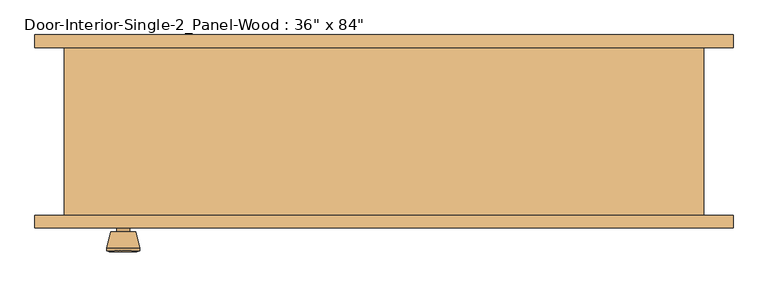
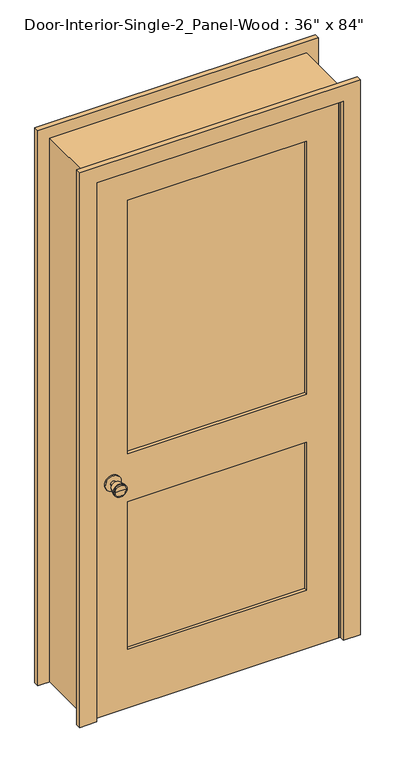
"""IFC4 building model written with IfcOpenShell, lengths in millimetres: door geometry."""

from ifc_helpers import new_model, si_unit, point, frame, frame_2d, origin, place, context, project, spatial, polyline, circle_curve, trimmed, segment, composite_curve, outline, extrude, faceted_brep, source, transform, mapped, element, save
from ifc_brep_helpers import plane_surface, cylinder_surface, revolved_surface, advanced_brep


def door_acb80719(model_context):
    return source(origin(), model_context, "Body", "SolidModel", [
        advanced_brep(
        [(-393.7, -82.9, 914.4), (-403.7, -82.9, 914.4), (-383.7, -82.9, 914.4), (-373.2241324, -33.9, 914.4), (-414.1758676, -33.9, 914.4), (-393.7, -33.9, 914.4), (-368.7, -35.7278681, 914.4), (-418.7, -35.7278681, 914.4), (-368.7, -39.1915463, 914.4), (-418.7, -39.1915463, 914.4), (-375.063764, -63.9, 914.4), (-412.336236, -63.9, 914.4), (-383.7, -63.9, 914.4), (-403.7, -63.9, 914.4)],
        [
            (0, 1),
            (1, 2, circle_curve(frame((-393.7, -82.9, 914.4), z_axis=(0.0, -1.0, 0.0), x_axis=(-1.0, 0.0, 0.0)), 10.0)),
            (2, 0),
            (2, 1, circle_curve(frame((-393.7, -82.9, 914.4), z_axis=(0.0, -1.0, 0.0), x_axis=(-1.0, 0.0, 0.0)), 10.0)),
            (3, 4, circle_curve(frame((-393.7, -33.9, 914.4), z_axis=(0.0, 1.0, 0.0), x_axis=(-1.0, 0.0, 0.0)), 20.4758676)),
            (4, 5),
            (5, 3),
            (4, 3, circle_curve(frame((-393.7, -33.9, 914.4), z_axis=(0.0, 1.0, 0.0), x_axis=(-1.0, 0.0, 0.0)), 20.4758676)),
            (6, 7, circle_curve(frame((-393.7, -35.7278681, 914.4), z_axis=(0.0, 1.0, 0.0), x_axis=(-1.0, 0.0, 0.0)), 25.0)),
            (7, 4),
            (3, 6),
            (7, 6, circle_curve(frame((-393.7, -35.7278681, 914.4), z_axis=(0.0, 1.0, 0.0), x_axis=(-1.0, 0.0, 0.0)), 25.0)),
            (8, 9, circle_curve(frame((-393.7, -39.1915463, 914.4), z_axis=(0.0, 1.0, 0.0), x_axis=(-1.0, 0.0, 0.0)), 25.0)),
            (9, 7),
            (6, 8),
            (9, 8, circle_curve(frame((-393.7, -39.1915463, 914.4), z_axis=(0.0, 1.0, 0.0), x_axis=(-1.0, 0.0, 0.0)), 25.0)),
            (10, 11, circle_curve(frame((-393.7, -63.9, 914.4), z_axis=(0.0, 1.0, 0.0), x_axis=(-1.0, 0.0, 0.0)), 18.636236)),
            (11, 9),
            (8, 10),
            (11, 10, circle_curve(frame((-393.7, -63.9, 914.4), z_axis=(0.0, 1.0, 0.0), x_axis=(-1.0, 0.0, 0.0)), 18.636236)),
            (12, 13, circle_curve(frame((-393.7, -63.9, 914.4), z_axis=(0.0, 1.0, 0.0), x_axis=(-1.0, 0.0, 0.0)), 10.0)),
            (13, 11),
            (10, 12),
            (13, 12, circle_curve(frame((-393.7, -63.9, 914.4), z_axis=(0.0, 1.0, 0.0), x_axis=(-1.0, 0.0, 0.0)), 10.0)),
            (1, 13),
            (12, 2),
        ],
        [
            plane_surface(frame((-393.7, -82.9, 914.4), z_axis=(0.0, -1.0, 0.0), x_axis=(-1.0, 0.0, 0.0))),
            plane_surface(frame((-393.7, -33.9, 914.4), z_axis=(0.0, 1.0, 0.0), x_axis=(-1.0, 0.0, 0.0))),
            revolved_surface(polyline([(-414.1758676, -33.9, 914.4), (-418.7, -35.7278681, 914.4)]), (-393.7, -82.9, 914.4), (0.0, -1.0, 0.0)),
            cylinder_surface(frame((-393.7, -82.9, 914.4), z_axis=(0.0, -1.0, 0.0), x_axis=(-1.0, 0.0, 0.0)), 25.0),
            revolved_surface(polyline([(-418.7, -39.1915463, 914.4), (-412.336236, -63.9, 914.4)]), (-393.7, -82.9, 914.4), (0.0, -1.0, 0.0)),
            plane_surface(frame((-393.7, -63.9, 914.4), z_axis=(0.0, -1.0, 0.0), x_axis=(-1.0, 0.0, 0.0))),
            cylinder_surface(frame((-393.7, -82.9, 914.4), z_axis=(0.0, -1.0, 0.0), x_axis=(-1.0, 0.0, 0.0)), 10.0),
        ],
        [
            (0, [[1, 2, 3]]),
            (0, [[-3, 4, -1]]),
            (1, [[5, 6, 7]]),
            (1, [[8, -7, -6]]),
            (2, [[9, 10, -5, 11]]),
            (2, [[12, -11, -8, -10]]),
            (3, [[13, 14, -9, 15]]),
            (3, [[16, -15, -12, -14]]),
            (4, [[17, 18, -13, 19]]),
            (4, [[20, -19, -16, -18]]),
            (5, [[21, 22, -17, 23]]),
            (5, [[24, -23, -20, -22]]),
            (6, [[-2, 25, -21, 26]]),
            (6, [[-4, -26, -24, -25]]),
        ],
    ),
        extrude(outline(composite_curve([segment(trimmed(circle_curve(frame_2d((914.4, -393.7)), 30.0), [point((914.4, -423.7))], [point((914.4, -363.7))], False, "CARTESIAN"), True, "CONTINUOUS"), segment(trimmed(circle_curve(frame_2d((914.4, -393.7)), 30.0), [point((914.4, -363.7))], [point((914.4, -423.7))], False, "CARTESIAN"), True, "CONTINUOUS")], self_intersect=False)), frame((0.0, -88.9, 0.0), z_axis=(0.0, 1.0, 0.0), x_axis=(0.0, 0.0, 1.0)), (0.0, 0.0, 1.0), 6.0),
        advanced_brep(
        [(-393.7, -129.825, 914.4), (-383.7, -129.825, 914.4), (-403.7, -129.825, 914.4), (-373.2241324, -178.825, 914.4), (-393.7, -178.825, 914.4), (-414.1758676, -178.825, 914.4), (-368.7, -176.9971319, 914.4), (-418.7, -176.9971319, 914.4), (-368.7, -173.5334537, 914.4), (-418.7, -173.5334537, 914.4), (-375.063764, -148.825, 914.4), (-412.336236, -148.825, 914.4), (-383.7, -148.825, 914.4), (-403.7, -148.825, 914.4)],
        [
            (0, 1),
            (1, 2, circle_curve(frame((-393.7, -129.825, 914.4), z_axis=(0.0, 1.0, 0.0), x_axis=(-1.0, 0.0, 0.0)), 10.0)),
            (2, 0),
            (2, 1, circle_curve(frame((-393.7, -129.825, 914.4), z_axis=(0.0, 1.0, 0.0), x_axis=(-1.0, 0.0, 0.0)), 10.0)),
            (3, 4),
            (4, 5),
            (5, 3, circle_curve(frame((-393.7, -178.825, 914.4), z_axis=(0.0, -1.0, 0.0), x_axis=(-1.0, 0.0, 0.0)), 20.4758676)),
            (3, 5, circle_curve(frame((-393.7, -178.825, 914.4), z_axis=(0.0, -1.0, 0.0), x_axis=(-1.0, 0.0, 0.0)), 20.4758676)),
            (6, 3),
            (5, 7),
            (7, 6, circle_curve(frame((-393.7, -176.9971319, 914.4), z_axis=(0.0, -1.0, 0.0), x_axis=(-1.0, 0.0, 0.0)), 25.0)),
            (6, 7, circle_curve(frame((-393.7, -176.9971319, 914.4), z_axis=(0.0, -1.0, 0.0), x_axis=(-1.0, 0.0, 0.0)), 25.0)),
            (8, 6),
            (7, 9),
            (9, 8, circle_curve(frame((-393.7, -173.5334537, 914.4), z_axis=(0.0, -1.0, 0.0), x_axis=(-1.0, 0.0, 0.0)), 25.0)),
            (8, 9, circle_curve(frame((-393.7, -173.5334537, 914.4), z_axis=(0.0, -1.0, 0.0), x_axis=(-1.0, 0.0, 0.0)), 25.0)),
            (10, 8),
            (9, 11),
            (11, 10, circle_curve(frame((-393.7, -148.825, 914.4), z_axis=(0.0, -1.0, 0.0), x_axis=(-1.0, 0.0, 0.0)), 18.636236)),
            (10, 11, circle_curve(frame((-393.7, -148.825, 914.4), z_axis=(0.0, -1.0, 0.0), x_axis=(-1.0, 0.0, 0.0)), 18.636236)),
            (12, 10),
            (11, 13),
            (13, 12, circle_curve(frame((-393.7, -148.825, 914.4), z_axis=(0.0, -1.0, 0.0), x_axis=(-1.0, 0.0, 0.0)), 10.0)),
            (12, 13, circle_curve(frame((-393.7, -148.825, 914.4), z_axis=(0.0, -1.0, 0.0), x_axis=(-1.0, 0.0, 0.0)), 10.0)),
            (1, 12),
            (13, 2),
        ],
        [
            plane_surface(frame((-393.7, -129.825, 914.4), z_axis=(0.0, 1.0, 0.0), x_axis=(-1.0, 0.0, 0.0))),
            plane_surface(frame((-393.7, -178.825, 914.4), z_axis=(0.0, -1.0, 0.0), x_axis=(-1.0, 0.0, 0.0))),
            revolved_surface(polyline([(-414.1758676, -178.825, 914.4), (-418.7, -176.9971319, 914.4)]), (-393.7, -129.825, 914.4), (0.0, 1.0, 0.0)),
            cylinder_surface(frame((-393.7, -129.825, 914.4), z_axis=(0.0, 1.0, 0.0), x_axis=(-1.0, 0.0, 0.0)), 25.0),
            revolved_surface(polyline([(-418.7, -173.5334537, 914.4), (-412.336236, -148.825, 914.4)]), (-393.7, -129.825, 914.4), (0.0, 1.0, 0.0)),
            plane_surface(frame((-393.7, -148.825, 914.4), z_axis=(0.0, 1.0, 0.0), x_axis=(-1.0, 0.0, 0.0))),
            cylinder_surface(frame((-393.7, -129.825, 914.4), z_axis=(0.0, 1.0, 0.0), x_axis=(-1.0, 0.0, 0.0)), 10.0),
        ],
        [
            (0, [[1, 2, 3]]),
            (0, [[-3, 4, -1]]),
            (1, [[5, 6, 7]]),
            (1, [[-6, -5, 8]]),
            (2, [[9, -7, 10, 11]]),
            (2, [[-10, -8, -9, 12]]),
            (3, [[13, -11, 14, 15]]),
            (3, [[-14, -12, -13, 16]]),
            (4, [[17, -15, 18, 19]]),
            (4, [[-18, -16, -17, 20]]),
            (5, [[21, -19, 22, 23]]),
            (5, [[-22, -20, -21, 24]]),
            (6, [[25, -23, 26, -2]]),
            (6, [[-26, -24, -25, -4]]),
        ],
    ),
        extrude(outline(composite_curve([segment(trimmed(circle_curve(frame_2d((914.4, -393.7)), 30.0), [point((914.4, -423.7))], [point((914.4, -363.7))], False, "CARTESIAN"), True, "CONTINUOUS"), segment(trimmed(circle_curve(frame_2d((914.4, -393.7)), 30.0), [point((914.4, -363.7))], [point((914.4, -423.7))], False, "CARTESIAN"), True, "CONTINUOUS")], self_intersect=False)), frame((0.0, -129.825, 0.0), z_axis=(0.0, 1.0, 0.0), x_axis=(0.0, 0.0, 1.0)), (0.0, 0.0, 1.0), 6.0),
        faceted_brep([(482.6, -123.825, 0.0), (457.2, -123.825, 0.0), (457.2, -88.9, 0.0), (444.5, -88.9, 0.0), (444.5, -53.975, 0.0), (457.2, -53.975, 0.0), (457.2, 130.175, 0.0), (482.6, 130.175, 0.0), (482.6, 130.175, 2159.0), (482.6, -123.825, 2159.0), (457.2, 130.175, 2133.6), (-457.2, 130.175, 2133.6), (-457.2, 130.175, 0.0), (-482.6, 130.175, 0.0), (-482.6, 130.175, 2159.0), (457.2, -53.975, 2133.6), (444.5, -53.975, 2120.9), (-444.5, -53.975, 2120.9), (-444.5, -53.975, 0.0), (-457.2, -53.975, 0.0), (-457.2, -53.975, 2133.6), (444.5, -88.9, 2120.9), (457.2, -88.9, 2133.6), (-457.2, -88.9, 2133.6), (-457.2, -88.9, 0.0), (-444.5, -88.9, 0.0), (-444.5, -88.9, 2120.9), (457.2, -123.825, 2133.6), (-482.6, -123.825, 2159.0), (-482.6, -123.825, 0.0), (-457.2, -123.825, 0.0), (-457.2, -123.825, 2133.6)], [[[0, 1, 2, 3, 4, 5, 6, 7]], [[7, 8, 9, 0]], [[6, 10, 11, 12, 13, 14, 8, 7]], [[5, 15, 10, 6]], [[4, 16, 17, 18, 19, 20, 15, 5]], [[3, 21, 16, 4]], [[2, 22, 23, 24, 25, 26, 21, 3]], [[1, 27, 22, 2]], [[0, 9, 28, 29, 30, 31, 27, 1]], [[8, 14, 28, 9]], [[15, 20, 11, 10]], [[21, 26, 17, 16]], [[27, 31, 23, 22]], [[29, 13, 12, 19, 18, 25, 24, 30]], [[14, 13, 29, 28]], [[20, 19, 12, 11]], [[26, 25, 18, 17]], [[31, 30, 24, 23]]]),
        extrude(outline(polyline([(2133.6, -457.2), (0.0, -457.2), (0.0, 457.2), (2133.6, 457.2), (2133.6, -457.2)]), holes=[polyline([(2014.5375, -336.55), (2014.5375, 336.55), (1009.65, 336.55), (1009.65, -336.55), (2014.5375, -336.55)]), polyline([(819.15, -336.55), (819.15, 336.55), (231.775, 336.55), (231.775, -336.55), (819.15, -336.55)])]), frame((0.0, -123.825, 0.0), z_axis=(0.0, 1.0, 0.0), x_axis=(0.0, 0.0, 1.0)), (0.0, 0.0, 1.0), 34.925),
        extrude(outline(polyline([(336.55, -100.5416667), (336.55, -112.1833333), (-336.55, -112.1833333), (-336.55, -100.5416667), (336.55, -100.5416667)])), frame((0.0, 0.0, 1009.65), z_axis=(0.0, 0.0, 1.0), x_axis=(1.0, 0.0, 0.0)), (0.0, 0.0, 1.0), 1004.8875),
        extrude(outline(polyline([(336.55, -100.5416667), (336.55, -112.1833333), (-336.55, -112.1833333), (-336.55, -100.5416667), (336.55, -100.5416667)])), frame((0.0, 0.0, 231.775), z_axis=(0.0, 0.0, 1.0), x_axis=(1.0, 0.0, 0.0)), (0.0, 0.0, 1.0), 587.375),
        extrude(outline(polyline([(0.0, 527.05), (2203.45, 527.05), (2203.45, -527.05), (0.0, -527.05), (0.0, -463.55), (2139.95, -463.55), (2139.95, 463.55), (0.0, 463.55), (0.0, 527.05)])), frame((0.0, -142.875, 0.0), z_axis=(0.0, 1.0, 0.0), x_axis=(0.0, 0.0, 1.0)), (0.0, 0.0, 1.0), 19.05),
        extrude(outline(polyline([(0.0, 527.05), (2203.45, 527.05), (2203.45, -527.05), (0.0, -527.05), (0.0, -463.55), (2139.95, -463.55), (2139.95, 463.55), (0.0, 463.55), (0.0, 527.05)])), frame((0.0, 130.175, 0.0), z_axis=(0.0, 1.0, 0.0), x_axis=(0.0, 0.0, 1.0)), (0.0, 0.0, 1.0), 19.05),
    ])


if __name__ == "__main__":
    model = new_model("IFC4")
    model_context = context("Model", 3, world=origin())
    ifc_project = project(units=[si_unit("LENGTHUNIT", "METRE", prefix="MILLI")], contexts=[model_context])
    site = spatial("IfcSite", under=ifc_project)
    building = spatial("IfcBuilding", under=site)
    placement = place(None, origin())
    door_shape = door_acb80719(model_context)
    element("IfcDoor", 1, ObjectType="Door-Interior-Single-2_Panel-Wood : 36\" x 84\"", at=placement, inside=building, context=model_context, shape_type="MappedRepresentation", body=[
        mapped(door_shape, transform((0.0, 0.0, 0.0), x_axis=(1.0, 0.0, 0.0), y_axis=(0.0, 1.0, 0.0), z_axis=(0.0, 0.0, 1.0))),
    ])
    save(model, "model.ifc")

# Revit data of these elements
# Type "Door-Interior-Single-2_Panel-Wood : 36\" x 84\""
#   Type Mark = "9"
#   Assembly Code = "C1020300"
#   Analytic Construction = "Wooden"
#   Top Rail = 0' - 4 11/16"
#   Thickness = 0' - 1 3/8"
#   Thermal Resistance (R) = 2.5876 (h·ft²·°F)/BTU
#   Swing Angle [instance default] = 90.00°
#   Stiles = 0' - 4 3/4"
#   Rough Width = 3' - 2"
#   Rough Height = 7' - 1"
#   Lock Rail = 0' - 7 1/2"
#   Height = 7' - 0"
#   Width = 3' - 0"
#   Heat Transfer Coefficient (U) = 0.3865 BTU/(h·ft²·°F)
#   Bottom Rail = 0' - 9 1/8"
#   Trim Material = Cherry
#   Panel Material = Cherry
#   Frame Material = Cherry
#   Door Handle Material = Aluminum
#   Visual Light Transmittance = 0
#   Solar Heat Gain Coefficient = 0
#   Wall Closure = (empty or 0)
#   Function = (empty or 0)
# Element 1 (IfcDoor, "Door-Interior-Single-2_Panel-Wood : 36\" x 84\"")
#   Materials on its faces: "Cherry", "Aluminum"
# Materials
#   "Cherry": class "Wood", colour RGB 226 177 128, transparency 0, Description = "Prunus Serotina", Cost = 0
#   "Aluminum": class "Metal", colour RGB 247 247 247, transparency 0, Description = "Aluminum 6061", Cost = 0
